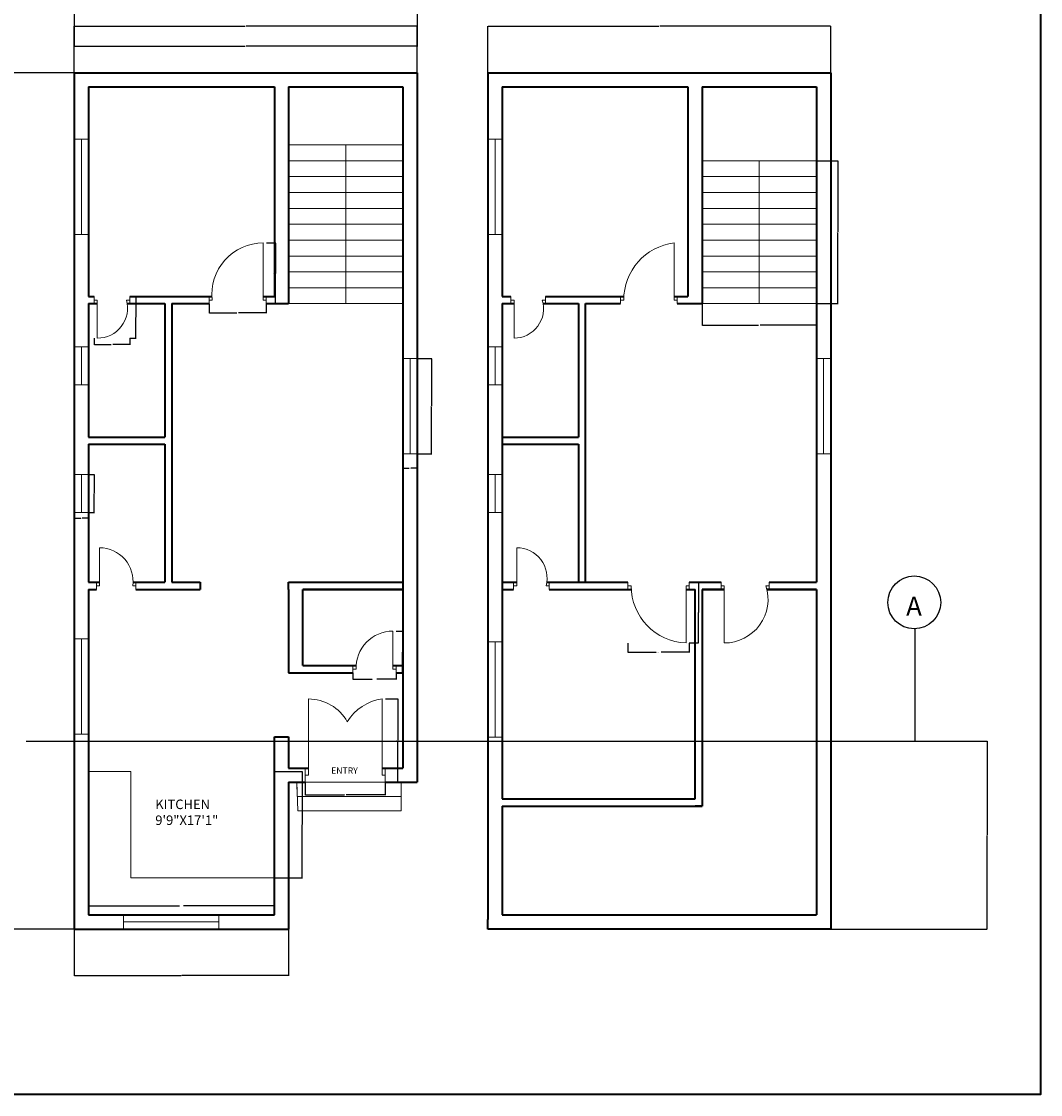
# Model space of a CAD drawing. Units: inches. Extents: x 2003 to 3241, y 1726 to 2849.
# Tile 6 of 7: x 2599 to 3241, y 1726 to 2402. Entities that reach past the tile are written whole.
import ezdxf

# ---------------------------------------------------------------- set-up
doc = ezdxf.new("R2010")
doc.units = ezdxf.units.IN
for name, color, linetype, lineweight in [('A-ANNO-DIMS', 2, 'Continuous', 18), ('A-ANNO-SYMB', 7, 'Continuous', 25), ('A-ANNO-TTLB', 7, 'Continuous', 35), ('A-AREA-IDEN', 7, 'Continuous', 18), ('A-DOOR', 3, 'Continuous', 18), ('A-FLOR-FIXT', 9, 'Continuous', 18), ('A-FLOR-STRS', 7, 'Continuous', 18), ('A-GLAZ', 4, 'Continuous', 18), ('A-WALL', 7, 'Continuous', 35)]:
    doc.layers.add(name, color=color, linetype=linetype, lineweight=lineweight)
doc.styles.get("Standard").update_dxf_attribs({"font": 'arial.ttf'})
doc.dimstyles.get("Standard").update_dxf_attribs({"dimtxt": 0.18, "dimasz": 0.18, "dimexe": 0.18, "dimexo": 0.0625, "dimgap": 0.09, "dimtad": 0, "dimtih": 1, "dimtoh": 1, "dimdec": 4, "dimzin": 0, "dimdsep": 46, "dimtxsty": 'Standard', "dimcen": 0.09, "dimadec": 0, "dimazin": 0, "dimtfac": 1, "dimtdec": 4, "dimtofl": 0, "dimtmove": 0, "dimatfit": 3, "dimfxl": 1, "dimtolj": 1, "dimtzin": 0, "dimarcsym": 0})

# ---------------------------------------------------------------- blocks, each defined once
blk = doc.blocks.new('WIN-60-1')
for p, q in [((0, 60), (9, 60)), ((9, 60), (4.5, 60)), ((4.5, 60), (4.5, 0)), ((4.5, 0), (0, 0)), ((0, 0), (9, 0))]:
    blk.add_line(p, q)
blk = doc.blocks.new('WIN-60-2')
for p, q in [((9, 60), (0, 60)), ((0, 60), (4.5, 60)), ((4.5, 60), (4.5, 0)), ((4.5, 0), (0, 0)), ((0, 0), (9, 0))]:
    blk.add_line(p, q)
blk = doc.blocks.new('WIN-24-1')
for p, q in [((0, 24), (9, 24)), ((9, 24), (4.5, 24)), ((4.5, 24), (4.5, 0)), ((4.5, 0), (0, 0)), ((0, 0), (9, 0))]:
    blk.add_line(p, q)
blk = doc.blocks.new('WIN-24-2')
for p, q in [((0, 24), (9, 24)), ((9, 24), (4.5, 24)), ((4.5, 24), (4.5, 0)), ((9, 0), (0, 0)), ((4.5, 0), (9, 0))]:
    blk.add_line(p, q)
blk = doc.blocks.new('WIN-60-HALL')
for p, q in [((0, 60), (9, 60)), ((9, 60), (4.5, 60)), ((4.5, 60), (4.5, 0)), ((4.5, 0), (0, 0)), ((0, 0), (9, 0)), ((9, 0), (9, 0))]:
    blk.add_line(p, q)
blk = doc.blocks.new('DOOR-ENTRY-PAIR')
for p, q in [((2, 4.5), (2, 52.5)), ((48.48, 4.5), (48.48, 52.5)), ((0, 9), (0, 0)), ((50.48, 9), (50.48, 0)), ((0, 4.5), (2, 4.5)), ((50.48, 4.5), (48.48, 4.5)), ((50.48, 0), (50.48, 4.5))]:
    blk.add_line(p, q)
for centre, radius, start, end in [((2, 24.35), 28.14, 29.23528, 90), ((52.39, 22.67), 30.08, 97.45976, 149.14255)]:
    blk.add_arc(centre, radius, start, end)
blk = doc.blocks.new('DOOR-POOJA')
for p, q in [((25.16, 2.25), (25.16, 26.25)), ((0, 4.5), (0, 0)), ((0, 0), (0, 2.25)), ((0, 2.25), (2, 2.25)), ((27.16, 2.25), (25.16, 2.25)), ((27.16, 4.5), (27.16, 0)), ((27.16, 0), (27.16, 2.25))]:
    blk.add_line(p, q)
blk.add_arc((25.16, 3.08), 23.17, 90, 182.04429)
blk = doc.blocks.new('DOOR-STORE')
for p, q in [((2, 2.25), (2, 26.25)), ((0, 4.5), (0, 0)), ((0, 0), (0, 2.25)), ((0, 2.25), (2, 2.25)), ((24.85, 2.25), (22.85, 2.25)), ((24.85, 4.5), (24.85, 0)), ((24.85, 0), (24.85, 2.25))]:
    blk.add_line(p, q)
blk.add_arc((2, 5.2), 21.05, 351.95387, 90)
blk = doc.blocks.new('DOOR-BEDROOM')
for p, q in [((34.02, 2.25), (34.02, 38.25)), ((0, 4.5), (0, 0)), ((0, 0), (0, 2.25)), ((0, 2.25), (2, 2.25)), ((36.02, 2.25), (34.02, 2.25)), ((36.02, 4.5), (36.02, 0)), ((36.02, 0), (36.02, 2.25))]:
    blk.add_line(p, q)
blk.add_arc((34.02, 6.01), 32.24, 90, 186.68896)
blk = doc.blocks.new('DOOR-BATH')
for p, q in [((0, 26.25), (0, 21.75)), ((0, 21.75), (0, 24)), ((0, 24), (2, 24)), ((2, 24), (2, 0)), ((22.43, 24), (20.43, 24)), ((22.43, 26.25), (22.43, 21.75)), ((22.43, 21.75), (22.43, 24))]:
    blk.add_line(p, q)
blk.add_arc((2, 19.08), 19.08, 270, 14.95524)
blk = doc.blocks.new('DOOR-BEDROOM-UPPER')
for p, q in [((33.76, 2.25), (33.76, 38.25)), ((0, 4.5), (0, 0)), ((0, 0), (0, 2.25)), ((0, 2.25), (2, 2.25)), ((35.76, 2.25), (33.76, 2.25)), ((35.76, 4.5), (35.76, 0)), ((35.76, 0), (35.76, 2.25))]:
    blk.add_line(p, q)
blk.add_arc((38.28, 2.25), 36.28, 97.16256, 180)
blk = doc.blocks.new('DOOR-TERRACE-BEDROOM')
for p, q in [((0, 38.25), (0, 33.75)), ((0, 33.75), (0, 36)), ((0, 36), (2, 36)), ((38.56, 36), (36.56, 36)), ((36.56, 36), (36.56, 0)), ((38.56, 38.25), (38.56, 33.75)), ((38.56, 33.75), (38.56, 36))]:
    blk.add_line(p, q)
blk.add_arc((38.03, 36), 36.03, 180, 267.65676)
blk = doc.blocks.new('DOOR-TERRACE')
for p, q in [((0, 38.25), (0, 33.75)), ((0, 36), (2, 36)), ((2, 36), (2, 0)), ((30.26, 36), (28.26, 36)), ((30.26, 38.25), (30.26, 33.75)), ((30.26, 33.75), (30.26, 36))]:
    blk.add_line(p, q)
blk.add_arc((2, 27.58), 27.58, 270, 17.78542)
blk = doc.blocks.new('STAIR-GROUND-RUN')
for p, q in [((0, 100), (72, 100)), ((36, 97.06), (36, 100)), ((36, 0), (36, 97.06)), ((0, 90), (72, 90)), ((0, 80), (72, 80)), ((0, 70), (72, 70)), ((0, 60), (72, 60)), ((0, 50), (72, 50)), ((0, 40), (72, 40)), ((0, 30), (72, 30)), ((0, 20), (72, 20)), ((0, 10), (72, 10)), ((0, 0), (72, 0))]:
    blk.add_line(p, q)
blk = doc.blocks.new('STAIR-UPPER-RUN')
for p, q in [((0, 90), (72, 90)), ((36, 0), (36, 90)), ((72, 90), (36, 90)), ((0, 80), (72, 80)), ((72, 80), (36, 80)), ((0, 70), (72, 70)), ((72, 70), (36, 70)), ((0, 60), (72, 60)), ((72, 60), (36, 60)), ((0, 50), (72, 50)), ((72, 50), (36, 50)), ((0, 40), (72, 40)), ((72, 40), (36, 40)), ((0, 30), (72, 30)), ((72, 30), (36, 30)), ((0, 20), (72, 20)), ((72, 20), (36, 20)), ((0, 10), (72, 10)), ((72, 10), (36, 10)), ((0, 0), (72, 0)), ((72, 0), (36, 0))]:
    blk.add_line(p, q)
blk = doc.blocks.new('STEPS-ENTRY')
for p, q in [((0.54, 0), (0, 18)), ((0, 18), (0.27, 9)), ((5.21, 18), (55.69, 18)), ((55.69, 18), (65.74, 18)), ((65.74, 18), (65.74, 0)), ((0.27, 9), (0.27, 9)), ((0.27, 9), (65.74, 9)), ((65.74, 0), (0.54, 0))]:
    blk.add_line(p, q)
blk = doc.blocks.new('COUNTER-KITCHEN-L')
for p, q in [((0, 67), (26.53, 67)), ((26.53, 67), (26.53, 0)), ((26.53, 0), (117, 0))]:
    blk.add_line(p, q)
blk = doc.blocks.new('*D24')
at = {"layer": 'A-ANNO-DIMS', "color": 0, "lineweight": -2, "transparency": 16777216}
for p, q in [((2641.51, 2116.82), (2645.22, 2116.82)), ((2645.04, 2116.64), (2645.04, 2105.01)), ((2645.04, 2093), (2645.04, 2104.64)), ((2641.51, 2092.82), (2645.22, 2092.82))]:
    blk.add_line(p, q, dxfattribs=at)
at = {"layer": 'A-ANNO-DIMS', "color": 0, "transparency": 16777216}
for points in [[(2645.01, 2116.64), (2645.07, 2116.64), (2645.04, 2116.82)], [(2645.01, 2093), (2645.07, 2093), (2645.04, 2092.82)]]:
    blk.add_solid(points, dxfattribs=at)
at = {"layer": 'Defpoints', "color": 0, "transparency": 16777216}
for p in [(2641.44, 2116.82), (2645.04, 2116.82), (2641.44, 2092.82)]:
    blk.add_point(p, dxfattribs=at)
at = {"layer": 'A-ANNO-DIMS', "color": 0, "transparency": 16777216, "insert": (2645.04, 2104.82), "char_height": 0.18, "attachment_point": 5}
blk.add_mtext('\\A1;WINDOW 24 TYP.', dxfattribs=at)
blk = doc.blocks.new('*D25')
at = {"layer": 'A-ANNO-DIMS', "color": 0, "lineweight": -2, "transparency": 16777216}
for p, q in [((2632.44, 2092.76), (2632.44, 2089.04)), ((2632.62, 2089.22), (2636.48, 2089.22)), ((2641.26, 2089.22), (2637.4, 2089.22)), ((2641.44, 2092.76), (2641.44, 2089.04))]:
    blk.add_line(p, q, dxfattribs=at)
at = {"layer": 'A-ANNO-DIMS', "color": 0, "transparency": 16777216}
for points in [[(2632.62, 2089.25), (2632.62, 2089.19), (2632.44, 2089.22)], [(2641.26, 2089.25), (2641.26, 2089.19), (2641.44, 2089.22)]]:
    blk.add_solid(points, dxfattribs=at)
at = {"layer": 'Defpoints', "color": 0, "transparency": 16777216}
for p in [(2632.44, 2092.82), (2641.44, 2092.82), (2641.44, 2089.22)]:
    blk.add_point(p, dxfattribs=at)
at = {"layer": 'A-ANNO-DIMS', "color": 0, "transparency": 16777216, "insert": (2636.94, 2089.22), "char_height": 0.18, "attachment_point": 5}
blk.add_mtext('\\A1;9 TYP.', dxfattribs=at)
blk = doc.blocks.new('*D34')
at = {"layer": 'A-ANNO-DIMS', "color": 0, "lineweight": -2, "transparency": 16777216}
for p, q in [((2848.51, 2189.81), (2857.62, 2189.81)), ((2857.44, 2189.63), (2857.44, 2160)), ((2857.44, 2129.99), (2857.44, 2159.63)), ((2848.51, 2129.81), (2857.62, 2129.81))]:
    blk.add_line(p, q, dxfattribs=at)
at = {"layer": 'A-ANNO-DIMS', "color": 0, "transparency": 16777216}
for points in [[(2857.41, 2189.63), (2857.47, 2189.63), (2857.44, 2189.81)], [(2857.41, 2129.99), (2857.47, 2129.99), (2857.44, 2129.81)]]:
    blk.add_solid(points, dxfattribs=at)
at = {"layer": 'Defpoints', "color": 0, "transparency": 16777216}
for p in [(2848.44, 2189.81), (2857.44, 2189.81), (2848.44, 2129.81)]:
    blk.add_point(p, dxfattribs=at)
at = {"layer": 'A-ANNO-DIMS', "color": 0, "transparency": 16777216, "insert": (2857.44, 2159.81), "char_height": 0.18, "attachment_point": 5}
blk.add_mtext('\\A1;WINDOW 60 TYP.', dxfattribs=at)
blk = doc.blocks.new('*D35')
at = {"layer": 'A-ANNO-DIMS', "color": 0, "lineweight": -2, "transparency": 16777216}
for p, q in [((2839.44, 2129.75), (2839.44, 2120.63)), ((2848.44, 2129.75), (2848.44, 2120.63)), ((2839.62, 2120.81), (2843.48, 2120.81)), ((2848.26, 2120.81), (2844.4, 2120.81))]:
    blk.add_line(p, q, dxfattribs=at)
at = {"layer": 'A-ANNO-DIMS', "color": 0, "transparency": 16777216}
for points in [[(2839.62, 2120.84), (2839.62, 2120.78), (2839.44, 2120.81)], [(2848.26, 2120.84), (2848.26, 2120.78), (2848.44, 2120.81)]]:
    blk.add_solid(points, dxfattribs=at)
at = {"layer": 'Defpoints', "color": 0, "transparency": 16777216}
for p in [(2839.44, 2129.81), (2848.44, 2129.81), (2848.44, 2120.81)]:
    blk.add_point(p, dxfattribs=at)
at = {"layer": 'A-ANNO-DIMS', "color": 0, "transparency": 16777216, "insert": (2843.94, 2120.81), "char_height": 0.18, "attachment_point": 5}
blk.add_mtext('\\A1;9 TYP.', dxfattribs=at)
blk = doc.blocks.new('*D36')
at = {"layer": 'A-ANNO-DIMS', "color": 0, "lineweight": -2, "transparency": 16777216}
for p, q in [((2828.4, 1975.41), (2836.39, 1975.41)), ((2836.21, 1975.23), (2836.21, 1949.35)), ((2836.21, 1923.09), (2836.21, 1948.98)), ((2828.4, 1922.91), (2836.39, 1922.91))]:
    blk.add_line(p, q, dxfattribs=at)
at = {"layer": 'A-ANNO-DIMS', "color": 0, "transparency": 16777216}
for points in [[(2836.18, 1975.23), (2836.24, 1975.23), (2836.21, 1975.41)], [(2836.18, 1923.09), (2836.24, 1923.09), (2836.21, 1922.91)]]:
    blk.add_solid(points, dxfattribs=at)
at = {"layer": 'Defpoints', "color": 0, "transparency": 16777216}
for p in [(2828.33, 1975.41), (2836.21, 1975.41), (2828.33, 1922.91)]:
    blk.add_point(p, dxfattribs=at)
at = {"layer": 'A-ANNO-DIMS', "color": 0, "transparency": 16777216, "insert": (2836.21, 1949.16), "char_height": 0.18, "attachment_point": 5}
blk.add_mtext('\\A1;ENTRY PAIR 53 TYP.', dxfattribs=at)
blk = doc.blocks.new('*D37')
at = {"layer": 'A-ANNO-DIMS', "color": 0, "lineweight": -2, "transparency": 16777216}
for p, q in [((2777.86, 1922.85), (2777.86, 1914.86)), ((2828.33, 1922.85), (2828.33, 1914.86)), ((2778.04, 1915.04), (2802.57, 1915.04)), ((2828.15, 1915.04), (2803.62, 1915.04))]:
    blk.add_line(p, q, dxfattribs=at)
at = {"layer": 'A-ANNO-DIMS', "color": 0, "transparency": 16777216}
for points in [[(2778.04, 1915.07), (2778.04, 1915.01), (2777.86, 1915.04)], [(2828.15, 1915.07), (2828.15, 1915.01), (2828.33, 1915.04)]]:
    blk.add_solid(points, dxfattribs=at)
at = {"layer": 'Defpoints', "color": 0, "transparency": 16777216}
for p in [(2777.86, 1922.91), (2828.33, 1922.91), (2828.33, 1915.04)]:
    blk.add_point(p, dxfattribs=at)
at = {"layer": 'A-ANNO-DIMS', "color": 0, "transparency": 16777216, "insert": (2803.1, 1915.04), "char_height": 0.18, "attachment_point": 5}
blk.add_mtext('\\A1;50 TYP.', dxfattribs=at)
blk = doc.blocks.new('*D38')
at = {"layer": 'A-ANNO-DIMS', "color": 0, "lineweight": -2, "transparency": 16777216}
for p, q in [((2807.94, 1991.85), (2807.94, 1987.66)), ((2808.12, 1987.84), (2820.13, 1987.84)), ((2834.92, 1987.84), (2822.92, 1987.84)), ((2835.1, 1991.85), (2835.1, 1987.66))]:
    blk.add_line(p, q, dxfattribs=at)
at = {"layer": 'A-ANNO-DIMS', "color": 0, "transparency": 16777216}
for points in [[(2808.12, 1987.87), (2808.12, 1987.81), (2807.94, 1987.84)], [(2834.92, 1987.87), (2834.92, 1987.81), (2835.1, 1987.84)]]:
    blk.add_solid(points, dxfattribs=at)
at = {"layer": 'Defpoints', "color": 0, "transparency": 16777216}
for p in [(2807.94, 1991.91), (2835.1, 1991.91), (2835.1, 1987.84)]:
    blk.add_point(p, dxfattribs=at)
at = {"layer": 'A-ANNO-DIMS', "color": 0, "transparency": 16777216, "insert": (2821.52, 1987.84), "char_height": 0.18, "attachment_point": 5}
blk.add_mtext('\\A1;POOJA DOOR 27 TYP.', dxfattribs=at)
blk = doc.blocks.new('*D39')
at = {"layer": 'A-ANNO-DIMS', "color": 0, "lineweight": -2, "transparency": 16777216}
for p, q in [((2835.16, 2018.16), (2839.36, 2018.16)), ((2839.18, 2017.98), (2839.18, 2005.22)), ((2839.18, 1992.09), (2839.18, 2004.86)), ((2835.16, 1991.91), (2839.36, 1991.91))]:
    blk.add_line(p, q, dxfattribs=at)
at = {"layer": 'A-ANNO-DIMS', "color": 0, "transparency": 16777216}
for points in [[(2839.15, 2017.98), (2839.21, 2017.98), (2839.18, 2018.16)], [(2839.15, 1992.09), (2839.21, 1992.09), (2839.18, 1991.91)]]:
    blk.add_solid(points, dxfattribs=at)
at = {"layer": 'Defpoints', "color": 0, "transparency": 16777216}
for p in [(2835.1, 2018.16), (2839.18, 2018.16), (2835.1, 1991.91)]:
    blk.add_point(p, dxfattribs=at)
at = {"layer": 'A-ANNO-DIMS', "color": 0, "transparency": 16777216, "insert": (2839.18, 2005.04), "char_height": 0.18, "attachment_point": 5}
blk.add_mtext('\\A1;26 TYP.', dxfattribs=at)
blk = doc.blocks.new('*D42')
at = {"layer": 'A-ANNO-DIMS', "color": 0, "lineweight": -2, "transparency": 16777216}
for p, q in [((2753.45, 2262.66), (2759.3, 2262.66)), ((2759.12, 2262.48), (2759.12, 2243.72)), ((2759.12, 2224.59), (2759.12, 2243.36)), ((2753.45, 2224.41), (2759.3, 2224.41))]:
    blk.add_line(p, q, dxfattribs=at)
at = {"layer": 'A-ANNO-DIMS', "color": 0, "transparency": 16777216}
for points in [[(2759.09, 2262.48), (2759.15, 2262.48), (2759.12, 2262.66)], [(2759.09, 2224.59), (2759.15, 2224.59), (2759.12, 2224.41)]]:
    blk.add_solid(points, dxfattribs=at)
at = {"layer": 'Defpoints', "color": 0, "transparency": 16777216}
for p in [(2753.39, 2262.66), (2759.12, 2262.66), (2753.39, 2224.41)]:
    blk.add_point(p, dxfattribs=at)
at = {"layer": 'A-ANNO-DIMS', "color": 0, "transparency": 16777216, "insert": (2759.12, 2243.54), "char_height": 0.18, "attachment_point": 5}
blk.add_mtext('\\A1;BEDROOM DOOR 38 TYP.', dxfattribs=at)
blk = doc.blocks.new('*D43')
at = {"layer": 'A-ANNO-DIMS', "color": 0, "lineweight": -2, "transparency": 16777216}
for p, q in [((2717.36, 2224.35), (2717.36, 2218.5)), ((2753.39, 2224.35), (2753.39, 2218.5)), ((2717.54, 2218.68), (2734.85, 2218.68)), ((2753.21, 2218.68), (2735.9, 2218.68))]:
    blk.add_line(p, q, dxfattribs=at)
at = {"layer": 'A-ANNO-DIMS', "color": 0, "transparency": 16777216}
for points in [[(2717.54, 2218.71), (2717.54, 2218.65), (2717.36, 2218.68)], [(2753.21, 2218.71), (2753.21, 2218.65), (2753.39, 2218.68)]]:
    blk.add_solid(points, dxfattribs=at)
at = {"layer": 'Defpoints', "color": 0, "transparency": 16777216}
for p in [(2717.36, 2224.41), (2753.39, 2224.41), (2753.39, 2218.68)]:
    blk.add_point(p, dxfattribs=at)
at = {"layer": 'A-ANNO-DIMS', "color": 0, "transparency": 16777216, "insert": (2735.37, 2218.68), "char_height": 0.18, "attachment_point": 5}
blk.add_mtext('\\A1;36 TYP.', dxfattribs=at)
blk = doc.blocks.new('*D44')
at = {"layer": 'A-ANNO-DIMS', "color": 0, "lineweight": -2, "transparency": 16777216}
for p, q in [((2667.4, 2228.91), (2671.46, 2228.91)), ((2671.28, 2228.73), (2671.28, 2215.97)), ((2671.28, 2202.84), (2671.28, 2215.61)), ((2667.4, 2202.66), (2671.46, 2202.66))]:
    blk.add_line(p, q, dxfattribs=at)
at = {"layer": 'A-ANNO-DIMS', "color": 0, "transparency": 16777216}
for points in [[(2671.25, 2228.73), (2671.31, 2228.73), (2671.28, 2228.91)], [(2671.25, 2202.84), (2671.31, 2202.84), (2671.28, 2202.66)]]:
    blk.add_solid(points, dxfattribs=at)
at = {"layer": 'Defpoints', "color": 0, "transparency": 16777216}
for p in [(2667.34, 2228.91), (2671.28, 2228.91), (2667.34, 2202.66)]:
    blk.add_point(p, dxfattribs=at)
at = {"layer": 'A-ANNO-DIMS', "color": 0, "transparency": 16777216, "insert": (2671.28, 2215.79), "char_height": 0.18, "attachment_point": 5}
blk.add_mtext('\\A1;BATH DOOR 26 TYP.', dxfattribs=at)
blk = doc.blocks.new('*D45')
at = {"layer": 'A-ANNO-DIMS', "color": 0, "lineweight": -2, "transparency": 16777216}
for p, q in [((2644.91, 2202.6), (2644.91, 2198.55)), ((2645.09, 2198.73), (2655.6, 2198.73)), ((2667.16, 2198.73), (2656.66, 2198.73)), ((2667.34, 2202.6), (2667.34, 2198.55))]:
    blk.add_line(p, q, dxfattribs=at)
at = {"layer": 'A-ANNO-DIMS', "color": 0, "transparency": 16777216}
for points in [[(2645.09, 2198.76), (2645.09, 2198.7), (2644.91, 2198.73)], [(2667.16, 2198.76), (2667.16, 2198.7), (2667.34, 2198.73)]]:
    blk.add_solid(points, dxfattribs=at)
at = {"layer": 'Defpoints', "color": 0, "transparency": 16777216}
for p in [(2644.91, 2202.66), (2667.34, 2202.66), (2667.34, 2198.73)]:
    blk.add_point(p, dxfattribs=at)
at = {"layer": 'A-ANNO-DIMS', "color": 0, "transparency": 16777216, "insert": (2656.13, 2198.73), "char_height": 0.18, "attachment_point": 5}
blk.add_mtext('\\A1;22 TYP.', dxfattribs=at)
blk = doc.blocks.new('*D48')
at = {"layer": 'A-ANNO-DIMS', "color": 0, "lineweight": -2, "transparency": 16777216}
for p, q in [((2981.22, 2010.6), (2981.22, 2004.7)), ((3019.78, 2010.6), (3019.78, 2004.7)), ((2981.4, 2004.88), (2998.88, 2004.88)), ((3019.6, 2004.88), (3002.12, 2004.88))]:
    blk.add_line(p, q, dxfattribs=at)
at = {"layer": 'A-ANNO-DIMS', "color": 0, "transparency": 16777216}
for points in [[(2981.4, 2004.91), (2981.4, 2004.85), (2981.22, 2004.88)], [(3019.6, 2004.91), (3019.6, 2004.85), (3019.78, 2004.88)]]:
    blk.add_solid(points, dxfattribs=at)
at = {"layer": 'Defpoints', "color": 0, "transparency": 16777216}
for p in [(2981.22, 2010.66), (3019.78, 2010.66), (3019.78, 2004.88)]:
    blk.add_point(p, dxfattribs=at)
at = {"layer": 'A-ANNO-DIMS', "color": 0, "transparency": 16777216, "insert": (3000.5, 2004.88), "char_height": 0.18, "attachment_point": 5}
blk.add_mtext('\\A1;BEDROOM DOOR 39 TYP.', dxfattribs=at)
blk = doc.blocks.new('*D49')
at = {"layer": 'A-ANNO-DIMS', "color": 0, "lineweight": -2, "transparency": 16777216}
for p, q in [((3019.84, 2048.91), (3025.74, 2048.91)), ((3025.56, 2048.73), (3025.56, 2029.97)), ((3025.56, 2010.84), (3025.56, 2029.61)), ((3019.84, 2010.66), (3025.74, 2010.66))]:
    blk.add_line(p, q, dxfattribs=at)
at = {"layer": 'A-ANNO-DIMS', "color": 0, "transparency": 16777216}
for points in [[(3025.53, 2048.73), (3025.59, 2048.73), (3025.56, 2048.91)], [(3025.53, 2010.84), (3025.59, 2010.84), (3025.56, 2010.66)]]:
    blk.add_solid(points, dxfattribs=at)
at = {"layer": 'Defpoints', "color": 0, "transparency": 16777216}
for p in [(3019.78, 2048.91), (3025.56, 2048.91), (3019.78, 2010.66)]:
    blk.add_point(p, dxfattribs=at)
at = {"layer": 'A-ANNO-DIMS', "color": 0, "transparency": 16777216, "insert": (3025.56, 2029.79), "char_height": 0.18, "attachment_point": 5}
blk.add_mtext('\\A1;38 TYP.', dxfattribs=at)
blk = doc.blocks.new('*D54')
at = {"layer": 'A-ANNO-DIMS', "color": 0, "lineweight": -2, "transparency": 16777216}
for p, q in [((3100.03, 2314.41), (3113.65, 2314.41)), ((3113.47, 2314.23), (3113.47, 2269.6)), ((3113.47, 2224.59), (3113.47, 2269.23)), ((3100.03, 2224.41), (3113.65, 2224.41))]:
    blk.add_line(p, q, dxfattribs=at)
at = {"layer": 'A-ANNO-DIMS', "color": 0, "transparency": 16777216}
for points in [[(3113.44, 2314.23), (3113.5, 2314.23), (3113.47, 2314.41)], [(3113.44, 2224.59), (3113.5, 2224.59), (3113.47, 2224.41)]]:
    blk.add_solid(points, dxfattribs=at)
at = {"layer": 'Defpoints', "color": 0, "transparency": 16777216}
for p in [(3099.97, 2314.41), (3113.47, 2314.41), (3099.97, 2224.41)]:
    blk.add_point(p, dxfattribs=at)
at = {"layer": 'A-ANNO-DIMS', "color": 0, "transparency": 16777216, "insert": (3113.47, 2269.41), "char_height": 0.18, "attachment_point": 5}
blk.add_mtext('\\A1;STAIR RUN 90 TYP.', dxfattribs=at)
blk = doc.blocks.new('*D55')
at = {"layer": 'A-ANNO-DIMS', "color": 0, "lineweight": -2, "transparency": 16777216}
for p, q in [((3027.97, 2224.35), (3027.97, 2210.73)), ((3099.97, 2224.35), (3099.97, 2210.73)), ((3028.15, 2210.91), (3063.44, 2210.91)), ((3099.79, 2210.91), (3064.49, 2210.91))]:
    blk.add_line(p, q, dxfattribs=at)
at = {"layer": 'A-ANNO-DIMS', "color": 0, "transparency": 16777216}
for points in [[(3028.15, 2210.94), (3028.15, 2210.88), (3027.97, 2210.91)], [(3099.79, 2210.94), (3099.79, 2210.88), (3099.97, 2210.91)]]:
    blk.add_solid(points, dxfattribs=at)
at = {"layer": 'Defpoints', "color": 0, "transparency": 16777216}
for p in [(3027.97, 2224.41), (3099.97, 2224.41), (3099.97, 2210.91)]:
    blk.add_point(p, dxfattribs=at)
at = {"layer": 'A-ANNO-DIMS', "color": 0, "transparency": 16777216, "insert": (3063.97, 2210.91), "char_height": 0.18, "attachment_point": 5}
blk.add_mtext('\\A1;72 TYP.', dxfattribs=at)
blk = doc.blocks.new('*D58')
at = {"layer": 'A-ANNO-DIMS', "color": 0, "lineweight": -2, "transparency": 16777216}
for p, q in [((2641.44, 1862.68), (2641.44, 1845.01)), ((2758.44, 1862.68), (2758.44, 1845.01)), ((2641.62, 1845.19), (2698.69, 1845.19)), ((2758.26, 1845.19), (2701.2, 1845.19))]:
    blk.add_line(p, q, dxfattribs=at)
at = {"layer": 'A-ANNO-DIMS', "color": 0, "transparency": 16777216}
for points in [[(2641.62, 1845.22), (2641.62, 1845.16), (2641.44, 1845.19)], [(2758.26, 1845.22), (2758.26, 1845.16), (2758.44, 1845.19)]]:
    blk.add_solid(points, dxfattribs=at)
at = {"layer": 'Defpoints', "color": 0, "transparency": 16777216}
for p in [(2641.44, 1862.74), (2758.44, 1862.74), (2758.44, 1845.19)]:
    blk.add_point(p, dxfattribs=at)
at = {"layer": 'A-ANNO-DIMS', "color": 0, "transparency": 16777216, "insert": (2699.94, 1845.19), "char_height": 0.18, "attachment_point": 5}
blk.add_mtext('\\A1;COUNTER 117 TYP.', dxfattribs=at)
blk = doc.blocks.new('*D59')
at = {"layer": 'A-ANNO-DIMS', "color": 0, "lineweight": -2, "transparency": 16777216}
for p, q in [((2758.51, 1929.74), (2776.17, 1929.74)), ((2775.99, 1929.56), (2775.99, 1896.42)), ((2775.99, 1862.92), (2775.99, 1896.06)), ((2758.51, 1862.74), (2776.17, 1862.74))]:
    blk.add_line(p, q, dxfattribs=at)
at = {"layer": 'A-ANNO-DIMS', "color": 0, "transparency": 16777216}
for points in [[(2775.96, 1929.56), (2776.02, 1929.56), (2775.99, 1929.74)], [(2775.96, 1862.92), (2776.02, 1862.92), (2775.99, 1862.74)]]:
    blk.add_solid(points, dxfattribs=at)
at = {"layer": 'Defpoints', "color": 0, "transparency": 16777216}
for p in [(2758.44, 1929.74), (2775.99, 1929.74), (2758.44, 1862.74)]:
    blk.add_point(p, dxfattribs=at)
at = {"layer": 'A-ANNO-DIMS', "color": 0, "transparency": 16777216, "insert": (2775.99, 1896.24), "char_height": 0.18, "attachment_point": 5}
blk.add_mtext('\\A1;67 TYP.', dxfattribs=at)
blk = doc.blocks.new('*D76')
at = {"layer": 'A-ANNO-DIMS', "color": 0, "lineweight": -2, "transparency": 16777216}
for p, q in [((2632.44, 2369.98), (2632.44, 2399.29)), ((2632.62, 2399.11), (2740.15, 2399.11)), ((2848.26, 2399.11), (2740.73, 2399.11)), ((2848.44, 2369.98), (2848.44, 2399.29))]:
    blk.add_line(p, q, dxfattribs=at)
at = {"layer": 'A-ANNO-DIMS', "color": 0, "transparency": 16777216}
for points in [[(2632.62, 2399.14), (2632.62, 2399.08), (2632.44, 2399.11)], [(2848.26, 2399.14), (2848.26, 2399.08), (2848.44, 2399.11)]]:
    blk.add_solid(points, dxfattribs=at)
at = {"layer": 'Defpoints', "color": 0, "transparency": 16777216}
for p in [(2848.44, 2399.11), (2632.44, 2369.91), (2848.44, 2369.91)]:
    blk.add_point(p, dxfattribs=at)
at = {"layer": 'A-ANNO-DIMS', "color": 0, "transparency": 16777216, "insert": (2740.44, 2399.11), "char_height": 0.18, "attachment_point": 5}
blk.add_mtext('\\A1;216', dxfattribs=at)
blk = doc.blocks.new('*D77')
at = {"layer": 'A-ANNO-DIMS', "color": 0, "lineweight": -2, "transparency": 16777216}
for p, q in [((2632.38, 2369.91), (2572.63, 2369.91)), ((2572.81, 2369.73), (2572.81, 2100.35)), ((2572.81, 1830.59), (2572.81, 2099.98)), ((2632.38, 1830.41), (2572.63, 1830.41))]:
    blk.add_line(p, q, dxfattribs=at)
at = {"layer": 'A-ANNO-DIMS', "color": 0, "transparency": 16777216}
for points in [[(2572.78, 2369.73), (2572.84, 2369.73), (2572.81, 2369.91)], [(2572.78, 1830.59), (2572.84, 1830.59), (2572.81, 1830.41)]]:
    blk.add_solid(points, dxfattribs=at)
at = {"layer": 'Defpoints', "color": 0, "transparency": 16777216}
for p in [(2572.81, 2369.91), (2632.44, 2369.91), (2632.44, 1830.41)]:
    blk.add_point(p, dxfattribs=at)
at = {"layer": 'A-ANNO-DIMS', "color": 0, "transparency": 16777216, "insert": (2572.81, 2100.16), "char_height": 0.18, "attachment_point": 5}
blk.add_mtext('\\A1;539.5', dxfattribs=at)
blk = doc.blocks.new('*D78')
at = {"layer": 'A-ANNO-DIMS', "color": 0, "lineweight": -2, "transparency": 16777216}
for p, q in [((2892.97, 2369.98), (2892.97, 2399.29)), ((2893.15, 2399.11), (3000.67, 2399.11)), ((3108.79, 2399.11), (3001.26, 2399.11)), ((3108.97, 2369.98), (3108.97, 2399.29))]:
    blk.add_line(p, q, dxfattribs=at)
at = {"layer": 'A-ANNO-DIMS', "color": 0, "transparency": 16777216}
for points in [[(2893.15, 2399.14), (2893.15, 2399.08), (2892.97, 2399.11)], [(3108.79, 2399.14), (3108.79, 2399.08), (3108.97, 2399.11)]]:
    blk.add_solid(points, dxfattribs=at)
at = {"layer": 'Defpoints', "color": 0, "transparency": 16777216}
for p in [(3108.97, 2399.11), (2892.97, 2369.91), (3108.97, 2369.91)]:
    blk.add_point(p, dxfattribs=at)
at = {"layer": 'A-ANNO-DIMS', "color": 0, "transparency": 16777216, "insert": (3000.97, 2399.11), "char_height": 0.18, "attachment_point": 5}
blk.add_mtext('\\A1;216', dxfattribs=at)
blk = doc.blocks.new('*D79')
at = {"layer": 'A-ANNO-DIMS', "color": 0, "lineweight": -2, "transparency": 16777216}
for p, q in [((2632.44, 1830.35), (2632.44, 1801.03)), ((2767.44, 1830.35), (2767.44, 1801.03)), ((2632.62, 1801.21), (2699.66, 1801.21)), ((2767.26, 1801.21), (2700.22, 1801.21))]:
    blk.add_line(p, q, dxfattribs=at)
at = {"layer": 'A-ANNO-DIMS', "color": 0, "transparency": 16777216}
for points in [[(2632.62, 1801.24), (2632.62, 1801.18), (2632.44, 1801.21)], [(2767.26, 1801.24), (2767.26, 1801.18), (2767.44, 1801.21)]]:
    blk.add_solid(points, dxfattribs=at)
at = {"layer": 'Defpoints', "color": 0, "transparency": 16777216}
for p in [(2632.44, 1830.41), (2767.44, 1830.41), (2767.44, 1801.21)]:
    blk.add_point(p, dxfattribs=at)
at = {"layer": 'A-ANNO-DIMS', "color": 0, "transparency": 16777216, "insert": (2699.94, 1801.21), "char_height": 0.18, "attachment_point": 5}
blk.add_mtext('\\A1;135', dxfattribs=at)
blk = doc.blocks.new('*D80')
at = {"layer": 'A-ANNO-DIMS', "color": 0, "lineweight": -2, "transparency": 16777216}
for p, q in [((3162.26, 1948.92), (3207.6, 1948.92)), ((3207.42, 1948.74), (3207.42, 1889.85)), ((3207.42, 1830.59), (3207.42, 1889.49)), ((3109.03, 1830.41), (3207.6, 1830.41))]:
    blk.add_line(p, q, dxfattribs=at)
at = {"layer": 'A-ANNO-DIMS', "color": 0, "transparency": 16777216}
for points in [[(3207.39, 1948.74), (3207.45, 1948.74), (3207.42, 1948.92)], [(3207.39, 1830.59), (3207.45, 1830.59), (3207.42, 1830.41)]]:
    blk.add_solid(points, dxfattribs=at)
at = {"layer": 'Defpoints', "color": 0, "transparency": 16777216}
for p in [(3162.2, 1948.92), (3207.42, 1948.92), (3108.97, 1830.41)]:
    blk.add_point(p, dxfattribs=at)
at = {"layer": 'A-ANNO-DIMS', "color": 0, "transparency": 16777216, "insert": (3207.42, 1889.67), "char_height": 0.18, "attachment_point": 5}
blk.add_mtext('\\A1;118.5', dxfattribs=at)
blk = doc.blocks.new('*D100')
at = {"layer": 'A-ANNO-DIMS', "color": 0, "lineweight": -2, "transparency": 16777216}
for p, q in [((2632.44, 2455.12), (2632.44, 2386.37)), ((2848.44, 2455.12), (2848.44, 2386.37)), ((2632.62, 2386.55), (2740.15, 2386.55)), ((2848.26, 2386.55), (2740.73, 2386.55))]:
    blk.add_line(p, q, dxfattribs=at)
at = {"layer": 'A-ANNO-DIMS', "color": 0, "transparency": 16777216}
for points in [[(2632.62, 2386.58), (2632.62, 2386.52), (2632.44, 2386.55)], [(2848.26, 2386.58), (2848.26, 2386.52), (2848.44, 2386.55)]]:
    blk.add_solid(points, dxfattribs=at)
at = {"layer": 'Defpoints', "color": 0, "transparency": 16777216}
for p in [(2632.44, 2455.18), (2848.44, 2455.18), (2848.44, 2386.55)]:
    blk.add_point(p, dxfattribs=at)
at = {"layer": 'A-ANNO-DIMS', "color": 0, "transparency": 16777216, "insert": (2740.44, 2386.55), "char_height": 0.18, "attachment_point": 5}
blk.add_mtext('\\A1;216', dxfattribs=at)

msp = doc.modelspace()

# ---------------------------------------------------------------- linework, layer by layer
at = {"layer": 'A-ANNO-SYMB'}
for p, q in [((3162.2025, 1948.9204), (3162.2025, 2019.5875)), ((2602.0116, 1948.9204), (3162.2025, 1948.9204))]:
    msp.add_line(p, q, dxfattribs=at)
msp.add_circle((3161.5693, 2036.2301), 16.6546, dxfattribs=at)
at = {"layer": 'A-ANNO-TTLB'}
msp.add_lwpolyline([(2003.2633, 2848.7261), (3241.1194, 2848.7261), (3241.1194, 1726.227), (2003.2633, 1726.227)], close=True, dxfattribs=at)
at = {"layer": 'A-DOOR'}
for p, q in [((2907.4483, 2228.9135), (2907.4483, 2224.4135)), ((2907.4483, 2224.4135), (2907.4483, 2226.6635)), ((2907.4483, 2226.6635), (2909.4483, 2226.6635)), ((2909.4483, 2226.6635), (2909.4483, 2202.6635)), ((2929.2324, 2226.6635), (2927.2324, 2226.6635)), ((2929.2324, 2228.9135), (2929.2324, 2224.4135)), ((2929.2324, 2224.4135), (2929.2324, 2226.6635)), ((2911.193, 2046.6635), (2911.193, 2070.6635)), ((2909.193, 2048.9135), (2909.193, 2044.4135)), ((2931.627, 2048.9135), (2931.627, 2044.4135)), ((2909.193, 2044.4135), (2909.193, 2046.6635)), ((2909.193, 2046.6635), (2911.193, 2046.6635)), ((2931.627, 2046.6635), (2929.627, 2046.6635)), ((2931.627, 2044.4135), (2931.627, 2046.6635))]:
    msp.add_line(p, q, dxfattribs=at)
for centre, radius, start, end in [((2909.4483, 2221.2526), 18.589, 270, 16.922821), ((2911.193, 2051.5841), 19.0794, 345.0544554, 90)]:
    msp.add_arc(centre, radius, start, end, dxfattribs=at)
at = {"layer": 'A-WALL'}
for p, q in [((2632.4427, 2369.9135), (2848.4427, 2369.9135)), ((2632.4427, 2369.9135), (2848.4427, 2369.9135)), ((2632.4427, 2369.9135), (2632.4427, 1830.4135)), ((2848.4427, 2369.9135), (2848.4427, 1922.9135)), ((2892.9651, 2369.9135), (3108.9651, 2369.9135)), ((2892.9651, 2369.9135), (2892.9651, 1836.4016)), ((3108.9651, 2369.9135), (3108.9651, 1836.4016)), ((2641.4427, 2360.9135), (2758.4427, 2360.9135)), ((2641.4427, 2360.9135), (2641.4427, 2228.9135)), ((2758.4427, 2360.9135), (2758.4427, 2228.9135)), ((2767.4427, 2360.9135), (2839.4427, 2360.9135)), ((2767.4427, 2360.9135), (2767.4427, 2228.9135)), ((2839.4427, 2360.9135), (2839.4427, 2228.9135)), ((2901.9651, 2360.9135), (3018.9651, 2360.9135)), ((2901.9651, 2360.9135), (2901.9651, 2228.9135)), ((3018.9651, 2360.9135), (3018.9651, 2228.9135)), ((3027.9651, 2360.9135), (3099.9651, 2360.9135)), ((3027.9651, 2360.9135), (3027.9651, 2224.4135)), ((3099.9651, 2360.9135), (3099.9651, 2048.9135)), ((2641.4427, 2228.9135), (2644.9106, 2228.9135)), ((2641.4427, 2224.4135), (2646.9106, 2224.4135)), ((2641.4427, 2224.4135), (2641.4427, 2140.4135)), ((2665.7993, 2224.4135), (2689.4427, 2224.4135)), ((2667.3413, 2228.9135), (2719.1782, 2228.9135)), ((2689.4427, 2224.4135), (2689.4427, 2140.4135)), ((2693.9427, 2224.4135), (2717.3625, 2224.4135)), ((2693.9427, 2224.4135), (2693.9427, 2048.9135)), ((2751.3872, 2228.9135), (2758.4427, 2228.9135)), ((2753.3872, 2224.4135), (2767.4427, 2224.4135)), ((2767.4427, 2228.9135), (2767.4427, 2224.4135)), ((2839.4427, 2228.9135), (2839.4427, 2224.4135)), ((2839.4427, 2224.4135), (2839.4427, 1931.9135)), ((2901.9651, 2228.9135), (2907.4483, 2228.9135)), ((2901.9651, 2224.4135), (2909.4483, 2224.4135)), ((2901.9651, 2224.4135), (2901.9651, 1912.4135)), ((2901.9651, 2224.4135), (2909.4483, 2224.4135)), ((2927.7666, 2224.4135), (2949.9651, 2224.4135)), ((2927.7666, 2224.4135), (2949.9651, 2224.4135)), ((2929.2324, 2228.9135), (2978.5921, 2228.9135)), ((2949.9651, 2224.4135), (2949.9651, 2140.4135)), ((2954.4651, 2224.4135), (2976.5223, 2224.4135)), ((2954.4651, 2048.9135), (2954.4651, 2224.4135)), ((3010.2814, 2228.9135), (3018.9651, 2228.9135)), ((3012.2814, 2224.4135), (3018.9651, 2224.4135)), ((3018.9651, 2224.4135), (3027.9651, 2224.4135)), ((2641.4427, 2140.4135), (2689.4427, 2140.4135)), ((2901.9651, 2140.4135), (2949.9651, 2140.4135)), ((2641.4427, 2135.9135), (2689.4427, 2135.9135)), ((2641.4427, 2135.9135), (2641.4427, 2048.9135)), ((2689.4427, 2135.9135), (2689.4427, 2048.9135)), ((2901.9651, 2135.9135), (2949.9651, 2135.9135)), ((2949.9651, 2135.9135), (2949.9651, 2048.9135)), ((2641.4427, 2048.9135), (2648.3658, 2048.9135)), ((2669.4074, 2048.9135), (2689.4427, 2048.9135)), ((2693.9427, 2048.9135), (2711.7947, 2048.9135)), ((2711.7947, 2048.9135), (2711.7947, 2044.4135)), ((2767.4427, 2048.9135), (2839.4427, 2048.9135)), ((2767.4427, 2044.4135), (2767.4427, 2048.9135)), ((2901.9651, 2048.9135), (2911.193, 2048.9135)), ((2930.0846, 2048.9135), (2981.2204, 2048.9135)), ((3019.7774, 2048.9135), (3039.8962, 2048.9135)), ((3070.1549, 2048.9135), (3099.9651, 2048.9135)), ((2641.4427, 2044.4135), (2646.3658, 2044.4135)), ((2641.4427, 2044.4135), (2641.4427, 1839.4135)), ((2671.2117, 2044.4135), (2693.9427, 2044.4135)), ((2693.9427, 2044.4135), (2711.7947, 2044.4135)), ((2767.4427, 2044.4135), (2767.4427, 1991.9135)), ((2776.4427, 2044.4135), (2839.4427, 2044.4135)), ((2839.4427, 2044.4135), (2776.4427, 2044.4135)), ((2776.4427, 1996.4135), (2776.4427, 2044.4135)), ((2901.9651, 2044.4135), (2909.193, 2044.4135)), ((2901.9651, 2044.4135), (2909.193, 2044.4135)), ((2931.627, 2044.4135), (2983.2907, 2044.4135)), ((2931.627, 2044.4135), (2954.4651, 2044.4135)), ((3017.7774, 2044.4135), (3023.4651, 2044.4135)), ((3023.4651, 1912.4135), (3023.4651, 2044.4135)), ((3027.9651, 2044.4135), (3041.8962, 2044.4135)), ((3041.8962, 2044.4135), (3027.9651, 2044.4135)), ((3027.9651, 2044.4135), (3027.9651, 1907.9135)), ((3068.773, 2044.4135), (3099.9651, 2044.4135)), ((3099.9651, 2044.4135), (3068.773, 2044.4135)), ((3099.9651, 2044.4135), (3099.9651, 1839.4135)), ((2776.4427, 1996.4135), (2809.9717, 1996.4135)), ((2833.1013, 1996.4135), (2839.4427, 1996.4135)), ((2767.4427, 1991.9135), (2807.9427, 1991.9135)), ((2767.4427, 1991.9135), (2776.4427, 1991.9135)), ((2835.1013, 1991.9135), (2839.4427, 1991.9135)), ((2758.4427, 1931.9135), (2758.4427, 1951.6161)), ((2758.4427, 1951.6161), (2767.4427, 1951.6161)), ((2767.4427, 1951.6161), (2767.4427, 1931.9135)), ((2758.4427, 1839.4135), (2758.4427, 1931.9135)), ((2767.4427, 1931.9135), (2779.8556, 1931.9135)), ((2826.3348, 1931.9135), (2839.4427, 1931.9135)), ((2767.4427, 1922.9135), (2777.8556, 1922.9135)), ((2767.4427, 1922.9135), (2767.4427, 1839.4135)), ((2828.3348, 1922.9135), (2848.4427, 1922.9135)), ((2901.9651, 1912.4135), (3023.4651, 1912.4135)), ((2901.9651, 1907.9135), (2901.9651, 1839.4135)), ((2901.9651, 1907.9135), (3027.9651, 1907.9135)), ((3027.9651, 1907.9135), (3023.4651, 1907.9135)), ((2641.4427, 1839.4135), (2758.4427, 1839.4135)), ((2641.4427, 1839.4135), (2758.4427, 1839.4135)), ((2767.4427, 1839.4135), (2767.4427, 1830.4135)), ((2901.9651, 1839.4135), (3099.9651, 1839.4135)), ((3108.9651, 1839.4135), (3108.9651, 1830.4135)), ((2892.9651, 1830.4135), (2892.9651, 1836.4016)), ((2632.4427, 1830.4135), (2767.4427, 1830.4135)), ((3108.9651, 1830.4135), (2892.9651, 1830.4135))]:
    msp.add_line(p, q, dxfattribs=at)

# ---------------------------------------------------------------- block references
at = {"layer": 'A-DOOR'}
for name, p in [('DOOR-BEDROOM', (2717.3623, 2224.414)), ('DOOR-BEDROOM-UPPER', (2976.5223, 2224.414)), ('DOOR-BATH', (2644.9103, 2202.664)), ('DOOR-STORE', (2646.3653, 2044.414)), ('DOOR-TERRACE-BEDROOM', (2981.2203, 2010.664)), ('DOOR-TERRACE', (3039.8963, 2010.664)), ('DOOR-POOJA', (2807.9423, 1991.914)), ('DOOR-ENTRY-PAIR', (2777.8553, 1922.914))]:
    msp.add_blockref(name, p, dxfattribs=at)
at = {"layer": 'A-FLOR-FIXT'}
msp.add_blockref('COUNTER-KITCHEN-L', (2641.4423, 1862.743), dxfattribs=at)
at = {"layer": 'A-FLOR-STRS'}
for name, p in [('STAIR-GROUND-RUN', (2767.4423, 2224.414)), ('STAIR-UPPER-RUN', (3027.9653, 2224.414)), ('STEPS-ENTRY', (2772.6493, 1904.914))]:
    msp.add_blockref(name, p, dxfattribs=at)
at = {"layer": 'A-GLAZ'}
for name, p in [('WIN-60-1', (2632.4423, 2268.0124)), ('WIN-60-1', (2892.9647, 2268.0124)), ('WIN-24-1', (2632.4423, 2173.279)), ('WIN-24-1', (2892.9647, 2173.279)), ('WIN-60-HALL', (2839.4423, 2129.815)), ('WIN-60-2', (3099.9653, 2129.815)), ('WIN-24-1', (2632.4423, 2092.8237)), ('WIN-24-2', (2892.9653, 2092.823)), ('WIN-60-1', (2632.4423, 1953.19)), ('WIN-60-1', (2892.9647, 1951.4154))]:
    msp.add_blockref(name, p, dxfattribs=at)
at = {"layer": 'A-GLAZ', "extrusion": (0, 0, -1), "zscale": -1, "rotation": 90}
msp.add_blockref('WIN-60-1', (-2663.4439, 1830.4131), dxfattribs=at)

# ---------------------------------------------------------------- texts
at = {"layer": 'A-ANNO-SYMB', "insert": (3156.427, 2039.823), "char_height": 12, "attachment_point": 1}
msp.add_mtext_dynamic_manual_height_columns('A', width=32.216662, gutter_width=12.5, heights=[0], dxfattribs=at)
at = {"layer": 'A-AREA-IDEN', "attachment_point": 1}
for s, width, insert, char_height in [('ENTRY', 32.095586, (2794.2392, 1932.274), 4), ('KITCHEN\\P9\'9"X17\'1"', 47.571551, (2683.4232, 1912.0195), 6)]:
    msp.add_mtext_dynamic_manual_height_columns(s, width=width, gutter_width=12.5, heights=[0], dxfattribs=dict(at, insert=insert, char_height=char_height))

# ---------------------------------------------------------------- dimensions: what is measured, and where the dimension line sits
at = {"layer": 'A-ANNO-DIMS'}
for base, p1, p2, picture, middle in [((2848.4427, 2386.5531), (2632.4427, 2455.181), (2848.4427, 2455.181), '*D100', (2740.4427, 2386.5531)), ((2848.4427, 2399.1135), (2632.4427, 2369.9135), (2848.4427, 2369.9135), '*D76', (2740.4427, 2399.1135)), ((3108.9651, 2399.1135), (2892.9651, 2369.9135), (3108.9651, 2369.9135), '*D78', (3000.9651, 2399.1135)), ((2767.4427, 1801.2135), (2632.4427, 1830.4135), (2767.4427, 1830.4135), '*D79', (2699.9427, 1801.2135))]:
    dim = msp.add_linear_dim(base=base, p1=p1, p2=p2, dimstyle='Standard', override={"dimdec": 0, "dimlfac": 1, "dimrnd": 0, "dimzin": 0, "dimdsep": 46, "dimlunit": 2}, dxfattribs=at)
    dim.commit()
    dim.dimension.update_dxf_attribs({"geometry": picture, "text_midpoint": middle})
for base, p1, p2, picture, middle in [((2572.8116, 2369.9135), (2632.4427, 1830.4135), (2632.4427, 2369.9135), '*D77', (2572.8116, 2100.1635)), ((3207.4239, 1948.9204), (3108.9651, 1830.4135), (3162.2025, 1948.9204), '*D80', (3207.4239, 1889.667))]:
    dim = msp.add_linear_dim(base=base, p1=p1, p2=p2, angle=90, dimstyle='Standard', override={"dimdec": 1, "dimlfac": 1, "dimrnd": 0, "dimzin": 0, "dimdsep": 46, "dimlunit": 2}, dxfattribs=at)
    dim.commit()
    dim.dimension.update_dxf_attribs({"geometry": picture, "text_midpoint": middle})
for base, p1, p2, text, picture, middle in [((3113.4651, 2314.4135), (3099.9651, 2224.4135), (3099.9651, 2314.4135), 'STAIR RUN <> TYP.', '*D54', (3113.4651, 2269.4135)), ((2759.1247, 2262.6635), (2753.3872, 2224.4135), (2753.3872, 2262.6635), 'BEDROOM DOOR <> TYP.', '*D42', (2759.1247, 2243.5385)), ((2671.2788, 2228.9135), (2667.3413, 2202.6635), (2667.3413, 2228.9135), 'BATH DOOR <> TYP.', '*D44', (2671.2788, 2215.7885)), ((2857.4427, 2189.8149), (2848.4427, 2129.8149), (2848.4427, 2189.8149), 'WINDOW <> TYP.', '*D34', (2857.4427, 2159.8149)), ((2645.0427, 2116.8234), (2641.4427, 2092.8234), (2641.4427, 2116.8234), 'WINDOW <> TYP.', '*D24', (2645.0427, 2104.8234)), ((3025.5609, 2048.9135), (3019.7774, 2010.6635), (3019.7774, 2048.9135), '<> TYP.', '*D49', (3025.5609, 2029.7885)), ((2839.1751, 2018.1635), (2835.1013, 1991.9135), (2835.1013, 2018.1635), '<> TYP.', '*D39', (2839.1751, 2005.0385)), ((2836.2097575949, 1975.4135172726), (2828.3347575949, 1922.9135172726), (2828.3347575949, 1975.4135172726), 'ENTRY PAIR <> TYP.', '*D36', (2836.2097575949, 1949.1635172726)), ((2775.9927, 1929.743), (2758.4427, 1862.7432), (2758.4427, 1929.743), '<> TYP.', '*D59', (2775.9927, 1896.2431))]:
    dim = msp.add_linear_dim(base=base, p1=p1, p2=p2, angle=90, text=text, dimstyle='Standard', override={"dimdec": 0, "dimlfac": 1, "dimrnd": 0, "dimzin": 0, "dimdsep": 46, "dimlunit": 2}, dxfattribs=at)
    dim.commit()
    dim.dimension.update_dxf_attribs({"geometry": picture, "text_midpoint": middle})
for base, p1, p2, text, picture, middle in [((2753.3872, 2218.676), (2717.3625, 2224.4135), (2753.3872, 2224.4135), '<> TYP.', '*D43', (2735.3749, 2218.676)), ((3099.9651, 2210.9135), (3027.9651, 2224.4135), (3099.9651, 2224.4135), '<> TYP.', '*D55', (3063.9651, 2210.9135)), ((2667.3413, 2198.726), (2644.9106, 2202.6635), (2667.3413, 2202.6635), '<> TYP.', '*D45', (2656.126, 2198.726)), ((2848.4427, 2120.8149), (2839.4427, 2129.8149), (2848.4427, 2129.8149), '<> TYP.', '*D35', (2843.9427, 2120.8149)), ((2641.4427, 2089.2234), (2632.4427, 2092.8234), (2641.4427, 2092.8234), '<> TYP.', '*D25', (2636.9427, 2089.2234)), ((3019.7774, 2004.88), (2981.2204, 2010.6635), (3019.7774, 2010.6635), 'BEDROOM DOOR <> TYP.', '*D48', (3000.4989, 2004.88)), ((2835.1013, 1987.8397), (2807.9427, 1991.9135), (2835.1013, 1991.9135), 'POOJA DOOR <> TYP.', '*D38', (2821.522, 1987.8397)), ((2828.3348, 1915.0385), (2777.8556, 1922.9135), (2828.3348, 1922.9135), '<> TYP.', '*D37', (2803.0952, 1915.0385)), ((2758.4427, 1845.1932), (2641.4427, 1862.7432), (2758.4427, 1862.7432), 'COUNTER <> TYP.', '*D58', (2699.9427, 1845.1932))]:
    dim = msp.add_linear_dim(base=base, p1=p1, p2=p2, text=text, dimstyle='Standard', override={"dimdec": 0, "dimlfac": 1, "dimrnd": 0, "dimzin": 0, "dimdsep": 46, "dimlunit": 2}, dxfattribs=at)
    dim.commit()
    dim.dimension.update_dxf_attribs({"geometry": picture, "text_midpoint": middle})

doc.saveas('drawing.dxf')
